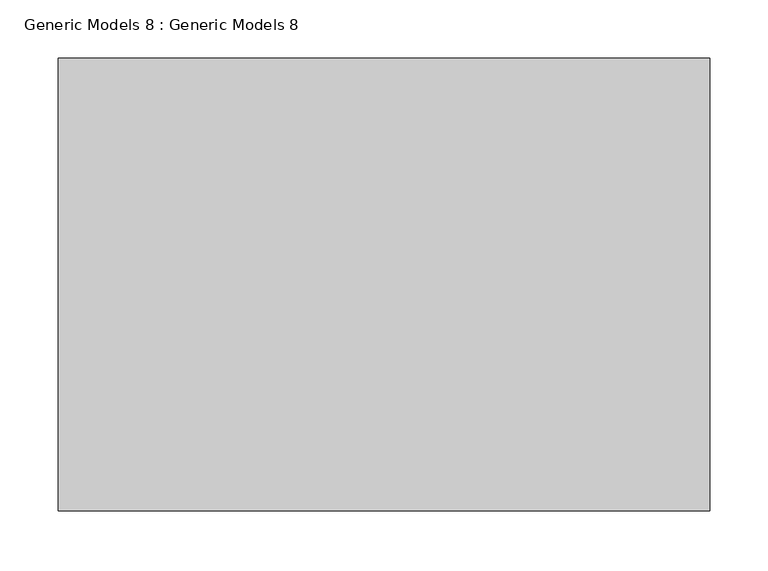
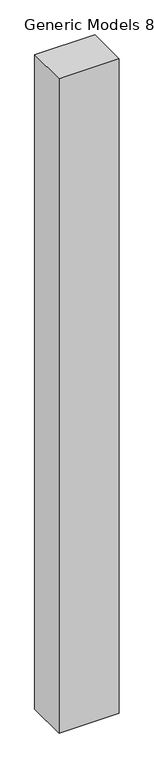
"""IFC4 building model written with IfcOpenShell, lengths in millimetres: proxy geometry, Generic Models 8 : Generic Models 8."""

from ifc_helpers import new_model, si_unit, origin, origin_with_axes, place, context, project, spatial, polyline, outline, extrude, source, transform, mapped, element, save


def generic_models_8_generic_models_8_60fedc48(model_context):
    return source(origin(), model_context, "Body", "SweptSolid", [
        extrude(outline(polyline([(609.2550588, -8520.3633093), (609.2550588, -8907.7133093), (52.3930105, -8907.7133093), (52.3930105, -8520.3633093), (609.2550588, -8520.3633093)])), origin_with_axes(), (0.0, 0.0, 1.0), 6402.8522437),
    ])


if __name__ == "__main__":
    model = new_model("IFC4")
    model_context = context("Model", 3, world=origin())
    ifc_project = project(units=[si_unit("LENGTHUNIT", "METRE", prefix="MILLI")], contexts=[model_context])
    site = spatial("IfcSite", under=ifc_project)
    building = spatial("IfcBuilding", under=site)
    placement = place(None, origin())
    generic_models_8_generic_models_8_shape = generic_models_8_generic_models_8_60fedc48(model_context)
    element("IfcBuildingElementProxy", 1, Name="Generic Models 8 : Generic Models 8", ObjectType="Generic Models 8 : Generic Models 8", at=placement, inside=building, context=model_context, shape_type="MappedRepresentation", body=[
        mapped(generic_models_8_generic_models_8_shape, transform((0.0, 0.0, 0.0), x_axis=(1.0, 0.0, 0.0), y_axis=(0.0, 1.0, 0.0), z_axis=(0.0, 0.0, 1.0))),
    ])
    save(model, "model.ifc")
